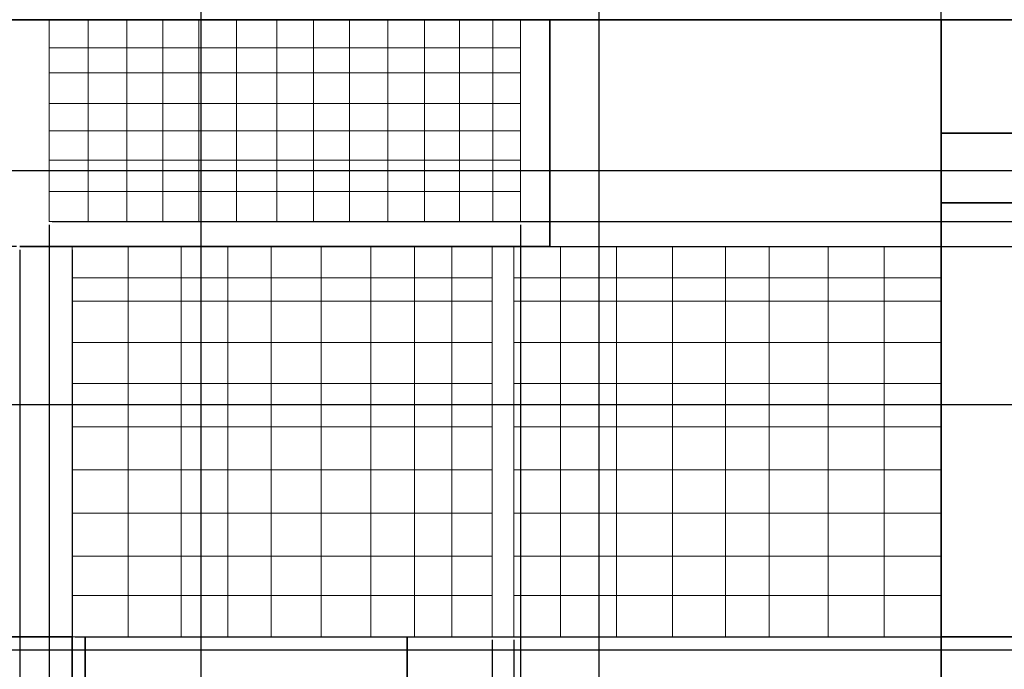
# Model space of a CAD drawing. Units: inches. Extents: x -10 to 130, y -32 to 34.
# Tile 15 of 22: x 70.9 to 90.41, y -6.87 to 6.01. Entities that reach past the tile are written whole.
import ezdxf

# ---------------------------------------------------------------- set-up
doc = ezdxf.new("R2010")
doc.units = ezdxf.units.IN
doc.header["$MEASUREMENT"] = 0
for name, color, linetype, lineweight in [('A-ANNO-DIMS', 2, 'Continuous', 18), ('A-ELEV', 7, 'Continuous', 35), ('A-GLAZ', 4, 'Continuous', 18)]:
    doc.layers.add(name, color=color, linetype=linetype, lineweight=lineweight)
doc.styles.get("Standard").update_dxf_attribs({"font": 'arial.ttf'})
doc.dimstyles.get("Standard").update_dxf_attribs({"dimtxt": 0.18, "dimasz": 0.18, "dimexe": 0.18, "dimexo": 0.0625, "dimgap": 0.09, "dimtad": 0, "dimtih": 1, "dimtoh": 1, "dimdec": 4, "dimzin": 0, "dimdsep": 46, "dimtxsty": 'Standard', "dimcen": 0.09, "dimadec": 0, "dimazin": 0, "dimtfac": 1, "dimtdec": 4, "dimtofl": 0, "dimtmove": 0, "dimatfit": 3, "dimfxl": 1, "dimtolj": 1, "dimtzin": 0, "dimarcsym": 0})

# ---------------------------------------------------------------- blocks, each defined once
blk = doc.blocks.new('*D2')
at = {"layer": 'A-ANNO-DIMS', "color": 0, "lineweight": -2, "transparency": 16777216}
for p, q in [((68.738, 27.199), (129.508, 27.199)), ((129.328, 27.019), (129.328, 3.074)), ((129.328, -21.234), (129.328, 2.71)), ((107.996, -21.414), (129.508, -21.414))]:
    blk.add_line(p, q, dxfattribs=at)
at = {"layer": 'A-ANNO-DIMS', "color": 0, "transparency": 16777216}
for points in [[(129.298, 27.019), (129.358, 27.019), (129.328, 27.199)], [(129.298, -21.234), (129.358, -21.234), (129.328, -21.414)]]:
    blk.add_solid(points, dxfattribs=at)
at = {"layer": 'Defpoints', "color": 0, "transparency": 16777216}
for p in [(68.676, 27.199), (129.328, 27.199), (107.933, -21.414)]:
    blk.add_point(p, dxfattribs=at)
at = {"layer": 'A-ANNO-DIMS', "color": 0, "transparency": 16777216, "insert": (129.328, 2.892), "char_height": 0.18, "attachment_point": 5}
blk.add_mtext('\\A1;48.61', dxfattribs=at)
blk = doc.blocks.new('*D33')
at = {"layer": 'A-ANNO-DIMS', "color": 0, "lineweight": -2, "transparency": 16777216}
for p, q in [((70.835, 1.511), (-9.564, 1.511)), ((-9.384, 1.331), (-9.384, 0.73)), ((-9.384, -0.234), (-9.384, 0.367)), ((31.909, -0.414), (-9.564, -0.414))]:
    blk.add_line(p, q, dxfattribs=at)
at = {"layer": 'A-ANNO-DIMS', "color": 0, "transparency": 16777216}
for points in [[(-9.414, 1.331), (-9.354, 1.331), (-9.384, 1.511)], [(-9.414, -0.234), (-9.354, -0.234), (-9.384, -0.414)]]:
    blk.add_solid(points, dxfattribs=at)
at = {"layer": 'Defpoints', "color": 0, "transparency": 16777216}
for p in [(-9.384, 1.511), (70.898, 1.511), (31.971, -0.414)]:
    blk.add_point(p, dxfattribs=at)
at = {"layer": 'A-ANNO-DIMS', "color": 0, "transparency": 16777216, "insert": (-9.384, 0.548), "char_height": 0.18, "attachment_point": 5}
blk.add_mtext('\\A1;1.92', dxfattribs=at)
blk = doc.blocks.new('*D34')
at = {"layer": 'A-ANNO-DIMS', "color": 0, "lineweight": -2, "transparency": 16777216}
for p, q in [((13.34, 6.007), (-9.564, 6.007)), ((-9.384, 5.827), (-9.384, 3.941)), ((-9.384, 1.691), (-9.384, 3.577)), ((70.835, 1.511), (-9.564, 1.511))]:
    blk.add_line(p, q, dxfattribs=at)
at = {"layer": 'A-ANNO-DIMS', "color": 0, "transparency": 16777216}
for points in [[(-9.414, 5.827), (-9.354, 5.827), (-9.384, 6.007)], [(-9.414, 1.691), (-9.354, 1.691), (-9.384, 1.511)]]:
    blk.add_solid(points, dxfattribs=at)
at = {"layer": 'Defpoints', "color": 0, "transparency": 16777216}
for p in [(-9.384, 6.007), (13.402, 6.007), (70.898, 1.511)]:
    blk.add_point(p, dxfattribs=at)
at = {"layer": 'A-ANNO-DIMS', "color": 0, "transparency": 16777216, "insert": (-9.384, 3.759), "char_height": 0.18, "attachment_point": 5}
blk.add_mtext('\\A1;4.497', dxfattribs=at)
blk = doc.blocks.new('*D48')
at = {"layer": 'A-ANNO-DIMS', "color": 0, "lineweight": -2, "transparency": 16777216}
for p, q in [((44.76, -13.293), (44.76, 33.879)), ((74.492, -13.293), (74.492, 33.879)), ((44.94, 33.699), (59.231, 33.699)), ((74.312, 33.699), (60.021, 33.699))]:
    blk.add_line(p, q, dxfattribs=at)
at = {"layer": 'A-ANNO-DIMS', "color": 0, "transparency": 16777216}
for points in [[(44.94, 33.729), (44.94, 33.669), (44.76, 33.699)], [(74.312, 33.729), (74.312, 33.669), (74.492, 33.699)]]:
    blk.add_solid(points, dxfattribs=at)
at = {"layer": 'Defpoints', "color": 0, "transparency": 16777216}
for p in [(74.492, 33.699), (44.76, -13.356), (74.492, -13.356)]:
    blk.add_point(p, dxfattribs=at)
at = {"layer": 'A-ANNO-DIMS', "color": 0, "transparency": 16777216, "insert": (59.626, 33.699), "char_height": 0.18, "attachment_point": 5}
blk.add_mtext('\\A1;29.73', dxfattribs=at)
blk = doc.blocks.new('*D60')
at = {"layer": 'A-ANNO-DIMS', "color": 0, "lineweight": -2, "transparency": 16777216}
for p, q in [((74.492, -13.293), (74.492, 33.879)), ((82.377, -15.202), (82.377, 33.879)), ((74.672, 33.699), (78.041, 33.699)), ((82.197, 33.699), (78.828, 33.699))]:
    blk.add_line(p, q, dxfattribs=at)
at = {"layer": 'A-ANNO-DIMS', "color": 0, "transparency": 16777216}
for points in [[(74.672, 33.729), (74.672, 33.669), (74.492, 33.699)], [(82.197, 33.729), (82.197, 33.669), (82.377, 33.699)]]:
    blk.add_solid(points, dxfattribs=at)
at = {"layer": 'Defpoints', "color": 0, "transparency": 16777216}
for p in [(82.377, 33.699), (74.492, -13.356), (82.377, -15.264)]:
    blk.add_point(p, dxfattribs=at)
at = {"layer": 'A-ANNO-DIMS', "color": 0, "transparency": 16777216, "insert": (78.435, 33.699), "char_height": 0.18, "attachment_point": 5}
blk.add_mtext('\\A1;7.885', dxfattribs=at)
blk = doc.blocks.new('*D66')
at = {"layer": 'A-ANNO-DIMS', "color": 0, "lineweight": -2, "transparency": 16777216}
for p, q in [((89.158, -16.844), (89.158, 33.879)), ((104.453, -13.219), (104.453, 33.879)), ((89.338, 33.699), (96.35, 33.699)), ((104.273, 33.699), (97.261, 33.699))]:
    blk.add_line(p, q, dxfattribs=at)
at = {"layer": 'A-ANNO-DIMS', "color": 0, "transparency": 16777216}
for points in [[(89.338, 33.729), (89.338, 33.669), (89.158, 33.699)], [(104.273, 33.729), (104.273, 33.669), (104.453, 33.699)]]:
    blk.add_solid(points, dxfattribs=at)
at = {"layer": 'Defpoints', "color": 0, "transparency": 16777216}
for p in [(104.453, 33.699), (104.453, -13.282), (89.158, -16.906)]:
    blk.add_point(p, dxfattribs=at)
at = {"layer": 'A-ANNO-DIMS', "color": 0, "transparency": 16777216, "insert": (96.805, 33.699), "char_height": 0.18, "attachment_point": 5}
blk.add_mtext('\\A1;15.295', dxfattribs=at)
blk = doc.blocks.new('*D76')
at = {"layer": 'A-ANNO-DIMS', "color": 0, "lineweight": -2, "transparency": 16777216}
for p, q in [((62.588, -6.485), (129.508, -6.485)), ((129.328, -6.665), (129.328, -8.76)), ((129.328, -11.218), (129.328, -9.123)), ((62.588, -11.398), (129.508, -11.398))]:
    blk.add_line(p, q, dxfattribs=at)
at = {"layer": 'A-ANNO-DIMS', "color": 0, "transparency": 16777216}
for points in [[(129.298, -6.665), (129.358, -6.665), (129.328, -6.485)], [(129.298, -11.218), (129.358, -11.218), (129.328, -11.398)]]:
    blk.add_solid(points, dxfattribs=at)
at = {"layer": 'Defpoints', "color": 0, "transparency": 16777216}
for p in [(62.526, -6.485), (129.328, -6.485), (62.526, -11.398)]:
    blk.add_point(p, dxfattribs=at)
at = {"layer": 'A-ANNO-DIMS', "color": 0, "transparency": 16777216, "insert": (129.328, -8.942), "char_height": 0.18, "attachment_point": 5}
blk.add_mtext('\\A1;4.913', dxfattribs=at)
blk = doc.blocks.new('*D77')
at = {"layer": 'A-ANNO-DIMS', "color": 0, "lineweight": -2, "transparency": 16777216}
for p, q in [((62.588, -1.618), (129.508, -1.618)), ((129.328, -1.798), (129.328, -3.87)), ((129.328, -6.305), (129.328, -4.234)), ((62.588, -6.485), (129.508, -6.485))]:
    blk.add_line(p, q, dxfattribs=at)
at = {"layer": 'A-ANNO-DIMS', "color": 0, "transparency": 16777216}
for points in [[(129.298, -1.798), (129.358, -1.798), (129.328, -1.618)], [(129.298, -6.305), (129.358, -6.305), (129.328, -6.485)]]:
    blk.add_solid(points, dxfattribs=at)
at = {"layer": 'Defpoints', "color": 0, "transparency": 16777216}
for p in [(62.526, -1.618), (129.328, -1.618), (62.526, -6.485)]:
    blk.add_point(p, dxfattribs=at)
at = {"layer": 'A-ANNO-DIMS', "color": 0, "transparency": 16777216, "insert": (129.328, -4.052), "char_height": 0.18, "attachment_point": 5}
blk.add_mtext('\\A1;4.866', dxfattribs=at)
blk = doc.blocks.new('*D78')
at = {"layer": 'A-ANNO-DIMS', "color": 0, "lineweight": -2, "transparency": 16777216}
for p, q in [((62.588, 3.018), (129.508, 3.018)), ((129.328, 2.838), (129.328, 0.882)), ((129.328, -1.438), (129.328, 0.518)), ((62.588, -1.618), (129.508, -1.618))]:
    blk.add_line(p, q, dxfattribs=at)
at = {"layer": 'A-ANNO-DIMS', "color": 0, "transparency": 16777216}
for points in [[(129.298, 2.838), (129.358, 2.838), (129.328, 3.018)], [(129.298, -1.438), (129.358, -1.438), (129.328, -1.618)]]:
    blk.add_solid(points, dxfattribs=at)
at = {"layer": 'Defpoints', "color": 0, "transparency": 16777216}
for p in [(62.526, 3.018), (129.328, 3.018), (62.526, -1.618)]:
    blk.add_point(p, dxfattribs=at)
at = {"layer": 'A-ANNO-DIMS', "color": 0, "transparency": 16777216, "insert": (129.328, 0.7), "char_height": 0.18, "attachment_point": 5}
blk.add_mtext('\\A1;4.64', dxfattribs=at)
blk = doc.blocks.new('*D79')
at = {"layer": 'A-ANNO-DIMS', "color": 0, "lineweight": -2, "transparency": 16777216}
for p, q in [((62.588, 7.736), (129.508, 7.736)), ((129.328, 7.556), (129.328, 5.559)), ((129.328, 3.198), (129.328, 5.195)), ((62.588, 3.018), (129.508, 3.018))]:
    blk.add_line(p, q, dxfattribs=at)
at = {"layer": 'A-ANNO-DIMS', "color": 0, "transparency": 16777216}
for points in [[(129.298, 7.556), (129.358, 7.556), (129.328, 7.736)], [(129.298, 3.198), (129.358, 3.198), (129.328, 3.018)]]:
    blk.add_solid(points, dxfattribs=at)
at = {"layer": 'Defpoints', "color": 0, "transparency": 16777216}
for p in [(62.526, 7.736), (129.328, 7.736), (62.526, 3.018)]:
    blk.add_point(p, dxfattribs=at)
at = {"layer": 'A-ANNO-DIMS', "color": 0, "transparency": 16777216, "insert": (129.328, 5.377), "char_height": 0.18, "attachment_point": 5}
blk.add_mtext('\\A1;4.718', dxfattribs=at)
blk = doc.blocks.new('*D139')
at = {"layer": 'A-ANNO-DIMS', "color": 0, "lineweight": -2, "transparency": 16777216}
for p, q in [((70.057, 6.643), (129.508, 6.643)), ((129.328, 6.463), (129.328, 6.187)), ((69.108, 6.007), (129.508, 6.007)), ((129.328, 6.007), (129.328, 5.827)), ((129.328, 5.827), (129.148, 5.827))]:
    blk.add_line(p, q, dxfattribs=at)
at = {"layer": 'A-ANNO-DIMS', "color": 0, "transparency": 16777216}
for points in [[(129.298, 6.463), (129.358, 6.463), (129.328, 6.643)], [(129.298, 6.187), (129.358, 6.187), (129.328, 6.007)]]:
    blk.add_solid(points, dxfattribs=at)
at = {"layer": 'Defpoints', "color": 0, "transparency": 16777216}
for p in [(69.995, 6.643), (69.045, 6.007), (129.328, 6.007)]:
    blk.add_point(p, dxfattribs=at)
at = {"layer": 'A-ANNO-DIMS', "color": 0, "transparency": 16777216, "insert": (128.754, 5.827), "char_height": 0.18, "attachment_point": 5}
blk.add_mtext('\\A1;0.636', dxfattribs=at)
blk = doc.blocks.new('*D151')
at = {"layer": 'A-ANNO-DIMS', "color": 0, "lineweight": -2, "transparency": 16777216}
for p, q in [((71.48, 1.942), (71.48, -28.129)), ((70.898, 1.448), (70.898, -28.129)), ((71.078, -27.949), (71.3, -27.949)), ((71.48, -27.949), (71.66, -27.949))]:
    blk.add_line(p, q, dxfattribs=at)
at = {"layer": 'A-ANNO-DIMS', "color": 0, "transparency": 16777216}
for points in [[(71.078, -27.919), (71.078, -27.979), (70.898, -27.949)], [(71.3, -27.919), (71.3, -27.979), (71.48, -27.949)]]:
    blk.add_solid(points, dxfattribs=at)
at = {"layer": 'Defpoints', "color": 0, "transparency": 16777216}
for p in [(71.48, 2.005), (70.898, 1.511), (71.48, -27.949)]:
    blk.add_point(p, dxfattribs=at)
at = {"layer": 'A-ANNO-DIMS', "color": 0, "transparency": 16777216, "insert": (72.053, -27.949), "char_height": 0.18, "attachment_point": 5}
blk.add_mtext('\\A1;0.582', dxfattribs=at)
blk = doc.blocks.new('*D152')
at = {"layer": 'A-ANNO-DIMS', "color": 0, "lineweight": -2, "transparency": 16777216}
for p, q in [((71.48, 1.942), (71.48, -28.129)), ((80.823, 1.942), (80.823, -28.129)), ((71.66, -27.949), (75.758, -27.949)), ((80.643, -27.949), (76.545, -27.949))]:
    blk.add_line(p, q, dxfattribs=at)
at = {"layer": 'A-ANNO-DIMS', "color": 0, "transparency": 16777216}
for points in [[(71.66, -27.919), (71.66, -27.979), (71.48, -27.949)], [(80.643, -27.919), (80.643, -27.979), (80.823, -27.949)]]:
    blk.add_solid(points, dxfattribs=at)
at = {"layer": 'Defpoints', "color": 0, "transparency": 16777216}
for p in [(71.48, 2.005), (80.823, 2.005), (80.823, -27.949)]:
    blk.add_point(p, dxfattribs=at)
at = {"layer": 'A-ANNO-DIMS', "color": 0, "transparency": 16777216, "insert": (76.152, -27.949), "char_height": 0.18, "attachment_point": 5}
blk.add_mtext('\\A1;9.343', dxfattribs=at)
blk = doc.blocks.new('*D153')
at = {"layer": 'A-ANNO-DIMS', "color": 0, "lineweight": -2, "transparency": 16777216}
for p, q in [((129.328, 2.185), (129.328, 2.365)), ((71.543, 2.005), (129.508, 2.005)), ((70.96, 1.511), (129.508, 1.511)), ((129.328, 1.331), (129.328, 1.151))]:
    blk.add_line(p, q, dxfattribs=at)
at = {"layer": 'A-ANNO-DIMS', "color": 0, "transparency": 16777216}
for points in [[(129.298, 2.185), (129.358, 2.185), (129.328, 2.005)], [(129.298, 1.331), (129.358, 1.331), (129.328, 1.511)]]:
    blk.add_solid(points, dxfattribs=at)
at = {"layer": 'Defpoints', "color": 0, "transparency": 16777216}
for p in [(71.48, 2.005), (70.898, 1.511), (129.328, 1.511)]:
    blk.add_point(p, dxfattribs=at)
at = {"layer": 'A-ANNO-DIMS', "color": 0, "transparency": 16777216, "insert": (129.328, 1.758), "char_height": 0.18, "attachment_point": 5}
blk.add_mtext('\\A1;0.494', dxfattribs=at)
blk = doc.blocks.new('*D154')
at = {"layer": 'A-ANNO-DIMS', "color": 0, "lineweight": -2, "transparency": 16777216}
for p, q in [((81.468, 6.007), (129.508, 6.007)), ((129.328, 5.827), (129.328, 3.941)), ((129.328, 1.691), (129.328, 3.577)), ((81.468, 1.511), (129.508, 1.511))]:
    blk.add_line(p, q, dxfattribs=at)
at = {"layer": 'A-ANNO-DIMS', "color": 0, "transparency": 16777216}
for points in [[(129.298, 5.827), (129.358, 5.827), (129.328, 6.007)], [(129.298, 1.691), (129.358, 1.691), (129.328, 1.511)]]:
    blk.add_solid(points, dxfattribs=at)
at = {"layer": 'Defpoints', "color": 0, "transparency": 16777216}
for p in [(81.405, 6.007), (129.328, 6.007), (81.405, 1.511)]:
    blk.add_point(p, dxfattribs=at)
at = {"layer": 'A-ANNO-DIMS', "color": 0, "transparency": 16777216, "insert": (129.328, 3.759), "char_height": 0.18, "attachment_point": 5}
blk.add_mtext('\\A1;4.497', dxfattribs=at)
blk = doc.blocks.new('*D155')
at = {"layer": 'A-ANNO-DIMS', "color": 0, "lineweight": -2, "transparency": 16777216}
for p, q in [((70.897993, 1.448166), (70.897993, -28.129305)), ((71.936707, 1.448166), (71.936707, -28.129305)), ((70.717993, -27.949305), (70.537993, -27.949305)), ((72.116707, -27.949305), (72.296707, -27.949305))]:
    blk.add_line(p, q, dxfattribs=at)
at = {"layer": 'A-ANNO-DIMS', "color": 0, "transparency": 16777216}
for points in [[(70.717993, -27.919305), (70.717993, -27.979305), (70.897993, -27.949305)], [(72.116707, -27.919305), (72.116707, -27.979305), (71.936707, -27.949305)]]:
    blk.add_solid(points, dxfattribs=at)
at = {"layer": 'Defpoints', "color": 0, "transparency": 16777216}
for p in [(70.897993, 1.510666), (71.936707, 1.510666), (71.936707, -27.949305)]:
    blk.add_point(p, dxfattribs=at)
at = {"layer": 'A-ANNO-DIMS', "color": 0, "transparency": 16777216, "insert": (71.41735, -27.949305), "char_height": 0.18, "attachment_point": 5}
blk.add_mtext('\\A1;1.039', dxfattribs=at)
blk = doc.blocks.new('*D156')
at = {"layer": 'A-ANNO-DIMS', "color": 0, "lineweight": -2, "transparency": 16777216}
for p, q in [((71.937, -6.284), (71.937, -28.129)), ((80.26, -6.284), (80.26, -28.129)), ((72.117, -27.949), (75.704, -27.949)), ((80.08, -27.949), (76.492, -27.949))]:
    blk.add_line(p, q, dxfattribs=at)
at = {"layer": 'A-ANNO-DIMS', "color": 0, "transparency": 16777216}
for points in [[(72.117, -27.919), (72.117, -27.979), (71.937, -27.949)], [(80.08, -27.919), (80.08, -27.979), (80.26, -27.949)]]:
    blk.add_solid(points, dxfattribs=at)
at = {"layer": 'Defpoints', "color": 0, "transparency": 16777216}
for p in [(71.937, -6.222), (80.26, -6.222), (80.26, -27.949)]:
    blk.add_point(p, dxfattribs=at)
at = {"layer": 'A-ANNO-DIMS', "color": 0, "transparency": 16777216, "insert": (76.098, -27.949), "char_height": 0.18, "attachment_point": 5}
blk.add_mtext('\\A1;8.323', dxfattribs=at)
blk = doc.blocks.new('*D157')
at = {"layer": 'A-ANNO-DIMS', "color": 0, "lineweight": -2, "transparency": 16777216}
for p, q in [((80.26, -6.284), (80.26, -28.129)), ((80.691, -6.284), (80.691, -28.129)), ((80.08, -27.949), (79.9, -27.949)), ((80.871, -27.949), (81.051, -27.949))]:
    blk.add_line(p, q, dxfattribs=at)
at = {"layer": 'A-ANNO-DIMS', "color": 0, "transparency": 16777216}
for points in [[(80.08, -27.919), (80.08, -27.979), (80.26, -27.949)], [(80.871, -27.919), (80.871, -27.979), (80.691, -27.949)]]:
    blk.add_solid(points, dxfattribs=at)
at = {"layer": 'Defpoints', "color": 0, "transparency": 16777216}
for p in [(80.26, -6.222), (80.691, -6.222), (80.691, -27.949)]:
    blk.add_point(p, dxfattribs=at)
at = {"layer": 'A-ANNO-DIMS', "color": 0, "transparency": 16777216, "insert": (81.444, -27.949), "char_height": 0.18, "attachment_point": 5}
blk.add_mtext('\\A1;0.432', dxfattribs=at)
blk = doc.blocks.new('*D158')
at = {"layer": 'A-ANNO-DIMS', "color": 0, "lineweight": -2, "transparency": 16777216}
for p, q in [((80.691, -6.284), (80.691, -28.129)), ((89.158, -6.284), (89.158, -28.129)), ((80.871, -27.949), (84.531, -27.949)), ((88.978, -27.949), (85.318, -27.949))]:
    blk.add_line(p, q, dxfattribs=at)
at = {"layer": 'A-ANNO-DIMS', "color": 0, "transparency": 16777216}
for points in [[(80.871, -27.919), (80.871, -27.979), (80.691, -27.949)], [(88.978, -27.919), (88.978, -27.979), (89.158, -27.949)]]:
    blk.add_solid(points, dxfattribs=at)
at = {"layer": 'Defpoints', "color": 0, "transparency": 16777216}
for p in [(80.691, -6.222), (89.158, -6.222), (89.158, -27.949)]:
    blk.add_point(p, dxfattribs=at)
at = {"layer": 'A-ANNO-DIMS', "color": 0, "transparency": 16777216, "insert": (84.925, -27.949), "char_height": 0.18, "attachment_point": 5}
blk.add_mtext('\\A1;8.466', dxfattribs=at)
blk = doc.blocks.new('*D159')
at = {"layer": 'A-ANNO-DIMS', "color": 0, "lineweight": -2, "transparency": 16777216}
for p, q in [((89.158, -6.284), (89.158, -28.129)), ((94.73, -6.284), (94.73, -28.129)), ((89.338, -27.949), (91.551, -27.949)), ((94.55, -27.949), (92.337, -27.949))]:
    blk.add_line(p, q, dxfattribs=at)
at = {"layer": 'A-ANNO-DIMS', "color": 0, "transparency": 16777216}
for points in [[(89.338, -27.919), (89.338, -27.979), (89.158, -27.949)], [(94.55, -27.919), (94.55, -27.979), (94.73, -27.949)]]:
    blk.add_solid(points, dxfattribs=at)
at = {"layer": 'Defpoints', "color": 0, "transparency": 16777216}
for p in [(89.158, -6.222), (94.73, -6.222), (94.73, -27.949)]:
    blk.add_point(p, dxfattribs=at)
at = {"layer": 'A-ANNO-DIMS', "color": 0, "transparency": 16777216, "insert": (91.944, -27.949), "char_height": 0.18, "attachment_point": 5}
blk.add_mtext('\\A1;5.572', dxfattribs=at)
blk = doc.blocks.new('*D160')
at = {"layer": 'A-ANNO-DIMS', "color": 0, "lineweight": -2, "transparency": 16777216}
for p, q in [((71.999, 1.511), (129.508, 1.511)), ((129.328, 1.331), (129.328, -2.174)), ((129.328, -6.042), (129.328, -2.538)), ((71.999, -6.222), (129.508, -6.222))]:
    blk.add_line(p, q, dxfattribs=at)
at = {"layer": 'A-ANNO-DIMS', "color": 0, "transparency": 16777216}
for points in [[(129.298, 1.331), (129.358, 1.331), (129.328, 1.511)], [(129.298, -6.042), (129.358, -6.042), (129.328, -6.222)]]:
    blk.add_solid(points, dxfattribs=at)
at = {"layer": 'Defpoints', "color": 0, "transparency": 16777216}
for p in [(71.937, 1.511), (71.937, -6.222), (129.328, -6.222)]:
    blk.add_point(p, dxfattribs=at)
at = {"layer": 'A-ANNO-DIMS', "color": 0, "transparency": 16777216, "insert": (129.328, -2.356), "char_height": 0.18, "attachment_point": 5}
blk.add_mtext('\\A1;7.732', dxfattribs=at)
blk = doc.blocks.new('*D168')
at = {"layer": 'A-ANNO-DIMS', "color": 0, "lineweight": -2, "transparency": 16777216}
for p, q in [((71.999, -6.222), (129.508, -6.222)), ((129.328, -6.402), (129.328, -7.024)), ((129.328, -8.009), (129.328, -7.387)), ((71.999, -8.189), (129.508, -8.189))]:
    blk.add_line(p, q, dxfattribs=at)
at = {"layer": 'A-ANNO-DIMS', "color": 0, "transparency": 16777216}
for points in [[(129.298, -6.402), (129.358, -6.402), (129.328, -6.222)], [(129.298, -8.009), (129.358, -8.009), (129.328, -8.189)]]:
    blk.add_solid(points, dxfattribs=at)
at = {"layer": 'Defpoints', "color": 0, "transparency": 16777216}
for p in [(71.937, -6.222), (71.937, -8.189), (129.328, -8.189)]:
    blk.add_point(p, dxfattribs=at)
at = {"layer": 'A-ANNO-DIMS', "color": 0, "transparency": 16777216, "insert": (129.328, -7.205), "char_height": 0.18, "attachment_point": 5}
blk.add_mtext('\\A1;1.967', dxfattribs=at)
blk = doc.blocks.new('*D169')
at = {"layer": 'A-ANNO-DIMS', "color": 0, "lineweight": -2, "transparency": 16777216}
for p, q in [((72.193, -6.284), (72.193, -28.129)), ((78.576, -6.284), (78.576, -28.129)), ((72.373, -27.949), (74.99, -27.949)), ((78.396, -27.949), (75.779, -27.949))]:
    blk.add_line(p, q, dxfattribs=at)
at = {"layer": 'A-ANNO-DIMS', "color": 0, "transparency": 16777216}
for points in [[(72.373, -27.919), (72.373, -27.979), (72.193, -27.949)], [(78.396, -27.919), (78.396, -27.979), (78.576, -27.949)]]:
    blk.add_solid(points, dxfattribs=at)
at = {"layer": 'Defpoints', "color": 0, "transparency": 16777216}
for p in [(72.193, -6.222), (78.576, -6.222), (78.576, -27.949)]:
    blk.add_point(p, dxfattribs=at)
at = {"layer": 'A-ANNO-DIMS', "color": 0, "transparency": 16777216, "insert": (75.384, -27.949), "char_height": 0.18, "attachment_point": 5}
blk.add_mtext('\\A1;6.383', dxfattribs=at)
blk = doc.blocks.new('*D172')
at = {"layer": 'A-ANNO-DIMS', "color": 0, "lineweight": -2, "transparency": 16777216}
for p, q in [((89.22, -6.222), (129.508, -6.222)), ((129.328, -6.402), (129.328, -6.85)), ((88.064, -7.03), (129.508, -7.03)), ((129.328, -7.21), (129.148, -7.21)), ((129.328, -7.03), (129.328, -7.21))]:
    blk.add_line(p, q, dxfattribs=at)
at = {"layer": 'A-ANNO-DIMS', "color": 0, "transparency": 16777216}
for points in [[(129.298, -6.402), (129.358, -6.402), (129.328, -6.222)], [(129.298, -6.85), (129.358, -6.85), (129.328, -7.03)]]:
    blk.add_solid(points, dxfattribs=at)
at = {"layer": 'Defpoints', "color": 0, "transparency": 16777216}
for p in [(89.158, -6.222), (88.002, -7.03), (129.328, -7.03)]:
    blk.add_point(p, dxfattribs=at)
at = {"layer": 'A-ANNO-DIMS', "color": 0, "transparency": 16777216, "insert": (128.754, -7.21), "char_height": 0.18, "attachment_point": 5}
blk.add_mtext('\\A1;0.808', dxfattribs=at)

msp = doc.modelspace()

# ---------------------------------------------------------------- linework, layer by layer
at = {"layer": 'A-ELEV'}
for p, q in [((98.6791, 6.0074), (69.0452, 6.0074)), ((81.4053, 1.5107), (81.4053, 6.0074)), ((89.1578, -6.2218), (89.1578, 6.0074)), ((94.7302, 3.7558), (89.1578, 3.7558)), ((94.7302, 2.375), (89.1578, 2.375)), ((70.898, 1.5107), (81.4053, 1.5107)), ((71.9367, -6.2218), (64.8443, -6.2218)), ((71.9367, -6.2218), (71.9367, -13.3558)), ((72.1928, -6.2218), (72.1928, -13.3558)), ((78.5759, -6.2218), (78.5759, -15.2645)), ((94.7302, -6.2218), (89.1578, -6.2218)), ((89.1578, -6.2218), (89.1578, -16.1883))]:
    msp.add_line(p, q, dxfattribs=at)
at = {"layer": 'A-GLAZ'}
for p, q in [((71.4801, 6.0074), (71.4801, 2.0049)), ((72.2515, 6.0074), (72.2515, 2.0049)), ((73.0228, 6.0074), (73.0228, 2.0049)), ((73.7359, 6.0074), (73.7359, 2.0049)), ((74.449, 6.0074), (74.449, 2.0049)), ((75.1913, 6.0074), (75.1913, 2.0049)), ((75.9917, 6.0074), (75.9917, 2.0049)), ((76.7194, 6.0074), (76.7194, 2.0049)), ((77.4325, 6.0074), (77.4325, 2.0049)), ((78.1893, 6.0074), (78.1893, 2.0049)), ((78.9169, 6.0074), (78.9169, 2.0049)), ((79.6155, 6.0074), (79.6155, 2.0049)), ((80.2704, 6.0074), (80.2704, 2.0049)), ((80.8232, 2.0049), (80.8232, 6.0074)), ((71.4801, 5.4499), (80.8232, 5.4499)), ((71.4801, 4.9557), (80.8232, 4.9557)), ((71.4801, 4.3452), (80.8232, 4.3452)), ((71.4801, 3.8074), (80.8232, 3.8074)), ((71.4801, 3.2259), (80.8232, 3.2259)), ((71.4801, 2.6009), (80.8232, 2.6009)), ((71.4801, 2.0049), (80.8232, 2.0049)), ((71.9367, 1.5107), (71.9367, -6.2218)), ((73.0465, 1.5107), (73.0465, -6.2218)), ((74.0946, 1.5107), (74.0946, -6.2218)), ((75.0194, 1.5107), (75.0194, -6.2218)), ((75.8825, 1.5107), (75.8825, -6.2218)), ((76.8689, 1.5107), (76.8689, -6.2218)), ((77.8554, 1.5107), (77.8554, -6.2218)), ((78.7185, 1.5107), (78.7185, -6.2218)), ((79.4584, 1.5107), (79.4584, -6.2218)), ((80.2599, 1.5107), (80.2599, -6.2218)), ((80.6914, 1.5107), (80.6914, -6.2218)), ((81.4053, 1.5107), (89.1578, 1.5107)), ((81.6162, 1.5107), (81.6162, -6.2218)), ((82.726, 1.5107), (82.726, -6.2218)), ((83.8357, 1.5107), (83.8357, -6.2218)), ((84.8838, 1.5107), (84.8838, -6.2218)), ((85.747, 1.5107), (85.747, -6.2218)), ((86.9184, 1.5107), (86.9184, -6.2218)), ((88.0281, 1.5107), (88.0281, -6.2218)), ((71.9367, 0.8941), (78.5759, 0.8941)), ((80.2599, 0.8941), (78.5759, 0.8941)), ((89.1578, 0.8941), (80.6914, 0.8941)), ((71.9367, 0.4275), (78.5759, 0.4275)), ((80.2599, 0.4275), (78.5759, 0.4275)), ((89.1578, 0.4275), (80.6914, 0.4275)), ((71.9367, -0.3891), (78.5759, -0.3891)), ((80.2599, -0.3891), (78.5759, -0.3891)), ((89.1578, -0.3891), (80.6914, -0.3891)), ((71.9367, -1.2057), (78.5759, -1.2057)), ((80.2599, -1.2057), (78.5759, -1.2057)), ((89.1578, -1.2057), (80.6914, -1.2057)), ((71.9367, -2.0611), (78.5759, -2.0611)), ((80.2599, -2.0611), (78.5759, -2.0611)), ((89.1578, -2.0611), (80.6914, -2.0611)), ((71.9367, -2.9166), (78.5759, -2.9166)), ((80.2599, -2.9166), (78.5759, -2.9166)), ((89.1578, -2.9166), (80.6914, -2.9166)), ((71.9367, -3.7721), (78.5759, -3.7721)), ((80.2599, -3.7721), (78.5759, -3.7721)), ((89.1578, -3.7721), (80.6914, -3.7721)), ((71.9367, -4.6275), (78.5759, -4.6275)), ((80.2599, -4.6275), (78.5759, -4.6275)), ((89.1578, -4.6275), (80.6914, -4.6275)), ((71.9367, -5.4052), (78.5759, -5.4052)), ((80.2599, -5.4052), (78.5759, -5.4052)), ((89.1578, -5.4052), (80.6914, -5.4052)), ((71.9367, -6.2218), (78.5759, -6.2218)), ((89.1578, -6.2218), (78.5759, -6.2218))]:
    msp.add_line(p, q, dxfattribs=at)

# ---------------------------------------------------------------- dimensions: what is measured, and where the dimension line sits
at = {"layer": 'A-ANNO-DIMS'}
for base, p1, p2, override, picture, middle in [((74.492, 33.6987), (44.76, -13.3558), (74.492, -13.3558), {"dimdec": 2, "dimlfac": 1, "dimrnd": 0, "dimzin": 0, "dimdsep": 46, "dimlunit": 2}, '*D48', (59.626, 33.6987)), ((82.377, 33.6987), (74.492, -13.3558), (82.377, -15.2645), {"dimdec": 3, "dimlfac": 1, "dimrnd": 0, "dimzin": 0, "dimdsep": 46, "dimlunit": 2}, '*D60', (78.4345, 33.6987)), ((104.4531, 33.6987), (89.1578, -16.9063), (104.4531, -13.2819), {"dimdec": 3, "dimlfac": 1, "dimrnd": 0, "dimzin": 0, "dimdsep": 46, "dimlunit": 2}, '*D66', (96.8055, 33.6987)), ((71.4801, -27.9493), (70.898, 1.5107), (71.4801, 2.0049), {"dimdec": 3, "dimlfac": 1, "dimrnd": 0, "dimzin": 0, "dimdsep": 46, "dimlunit": 2}, '*D151', (72.0529, -27.9493)), ((80.8232, -27.9493), (71.4801, 2.0049), (80.8232, 2.0049), {"dimdec": 3, "dimlfac": 1, "dimrnd": 0, "dimzin": 0, "dimdsep": 46, "dimlunit": 2}, '*D152', (76.1517, -27.9493)), ((71.9367, -27.9493), (70.898, 1.5107), (71.9367, 1.5107), {"dimdec": 3, "dimlfac": 1, "dimrnd": 0, "dimzin": 0, "dimdsep": 46, "dimlunit": 2}, '*D155', (71.4173, -27.9493)), ((80.2599, -27.9493), (71.9367, -6.2218), (80.2599, -6.2218), {"dimdec": 3, "dimlfac": 1, "dimrnd": 0, "dimzin": 0, "dimdsep": 46, "dimlunit": 2}, '*D156', (76.0983, -27.9493)), ((78.5759, -27.9493), (72.1928, -6.2218), (78.5759, -6.2218), {"dimdec": 3, "dimlfac": 1, "dimrnd": 0, "dimzin": 0, "dimdsep": 46, "dimlunit": 2}, '*D169', (75.3844, -27.9493)), ((80.69143, -27.9493), (80.25986, -6.22179), (80.69143, -6.22179), {"dimdec": 3, "dimlfac": 1, "dimrnd": 0, "dimzin": 0, "dimdsep": 46, "dimlunit": 2}, '*D157', (81.44421, -27.9493)), ((89.1578, -27.9493), (80.6914, -6.2218), (89.1578, -6.2218), {"dimdec": 3, "dimlfac": 1, "dimrnd": 0, "dimzin": 0, "dimdsep": 46, "dimlunit": 2}, '*D158', (84.9246, -27.9493)), ((94.7302, -27.9493), (89.1578, -6.2218), (94.7302, -6.2218), {"dimdec": 3, "dimlfac": 1, "dimrnd": 0, "dimzin": 0, "dimdsep": 46, "dimlunit": 2}, '*D159', (91.944, -27.9493))]:
    dim = msp.add_linear_dim(base=base, p1=p1, p2=p2, dimstyle='Standard', override=override, dxfattribs=at)
    dim.commit()
    dim.dimension.update_dxf_attribs({"geometry": picture, "text_midpoint": middle})
for base, p1, p2, override, picture, middle in [((129.3277, 27.1987), (107.9333, -21.4145), (68.6759, 27.1987), {"dimdec": 2, "dimlfac": 1, "dimrnd": 0, "dimzin": 0, "dimdsep": 46, "dimlunit": 2}, '*D2', (129.3277, 2.8921)), ((129.3277, 7.7364), (62.5256, 3.0181), (62.5256, 7.7364), {"dimdec": 3, "dimlfac": 1, "dimrnd": 0, "dimzin": 0, "dimdsep": 46, "dimlunit": 2}, '*D79', (129.3277, 5.3773)), ((129.3277, 6.0074), (69.9946, 6.6433), (69.0452, 6.0074), {"dimdec": 3, "dimlfac": 1, "dimrnd": 0, "dimzin": 0, "dimdsep": 46, "dimlunit": 2}, '*D139', (128.754, 5.8274)), ((-9.3836, 6.0074), (70.898, 1.5107), (13.4021, 6.0074), {"dimdec": 3, "dimlfac": 1, "dimrnd": 0, "dimzin": 0, "dimdsep": 46, "dimlunit": 2}, '*D34', (-9.3836, 3.7591)), ((129.3277, 6.0074), (81.4053, 1.5107), (81.4053, 6.0074), {"dimdec": 3, "dimlfac": 1, "dimrnd": 0, "dimzin": 0, "dimdsep": 46, "dimlunit": 2}, '*D154', (129.3277, 3.7591)), ((129.3277, 3.0181), (62.5256, -1.6184), (62.5256, 3.0181), {"dimdec": 2, "dimlfac": 1, "dimrnd": 0, "dimzin": 0, "dimdsep": 46, "dimlunit": 2}, '*D78', (129.3277, 0.6998)), ((129.3277, 1.5107), (71.4801, 2.0049), (70.898, 1.5107), {"dimdec": 3, "dimlfac": 1, "dimrnd": 0, "dimzin": 0, "dimdsep": 46, "dimlunit": 2}, '*D153', (129.3277, 1.7578)), ((-9.3836, 1.5107), (31.9712, -0.4138), (70.898, 1.5107), {"dimdec": 2, "dimlfac": 1, "dimrnd": 0, "dimzin": 0, "dimdsep": 46, "dimlunit": 2}, '*D33', (-9.3836, 0.5484)), ((129.32767, -6.22179), (71.93671, 1.51067), (71.93671, -6.22179), {"dimdec": 3, "dimlfac": 1, "dimrnd": 0, "dimzin": 0, "dimdsep": 46, "dimlunit": 2}, '*D160', (129.32767, -2.35556)), ((129.32767, -1.61843), (62.52563, -6.48486), (62.52563, -1.61843), {"dimdec": 3, "dimlfac": 1, "dimrnd": 0, "dimzin": 0, "dimdsep": 46, "dimlunit": 2}, '*D77', (129.32767, -4.05165)), ((129.3277, -8.1891), (71.9367, -6.2218), (71.9367, -8.1891), {"dimdec": 3, "dimlfac": 1, "dimrnd": 0, "dimzin": 0, "dimdsep": 46, "dimlunit": 2}, '*D168', (129.3277, -7.2054)), ((129.3277, -7.0301), (89.1578, -6.2218), (88.0017, -7.0301), {"dimdec": 3, "dimlfac": 1, "dimrnd": 0, "dimzin": 0, "dimdsep": 46, "dimlunit": 2}, '*D172', (128.7538, -7.2101)), ((129.3277, -6.4849), (62.5256, -11.3982), (62.5256, -6.4849), {"dimdec": 3, "dimlfac": 1, "dimrnd": 0, "dimzin": 0, "dimdsep": 46, "dimlunit": 2}, '*D76', (129.3277, -8.9415))]:
    dim = msp.add_linear_dim(base=base, p1=p1, p2=p2, angle=90, dimstyle='Standard', override=override, dxfattribs=at)
    dim.commit()
    dim.dimension.update_dxf_attribs({"geometry": picture, "text_midpoint": middle})

doc.saveas('drawing.dxf')
